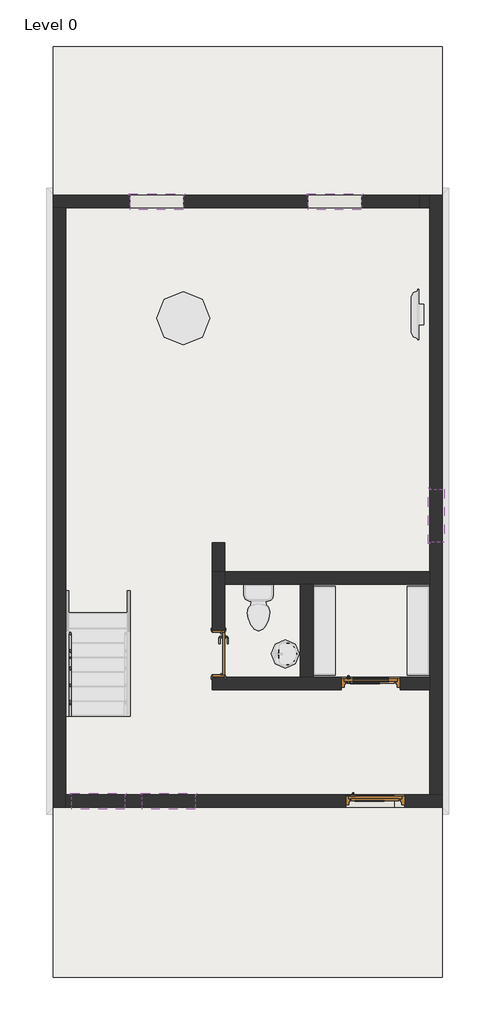
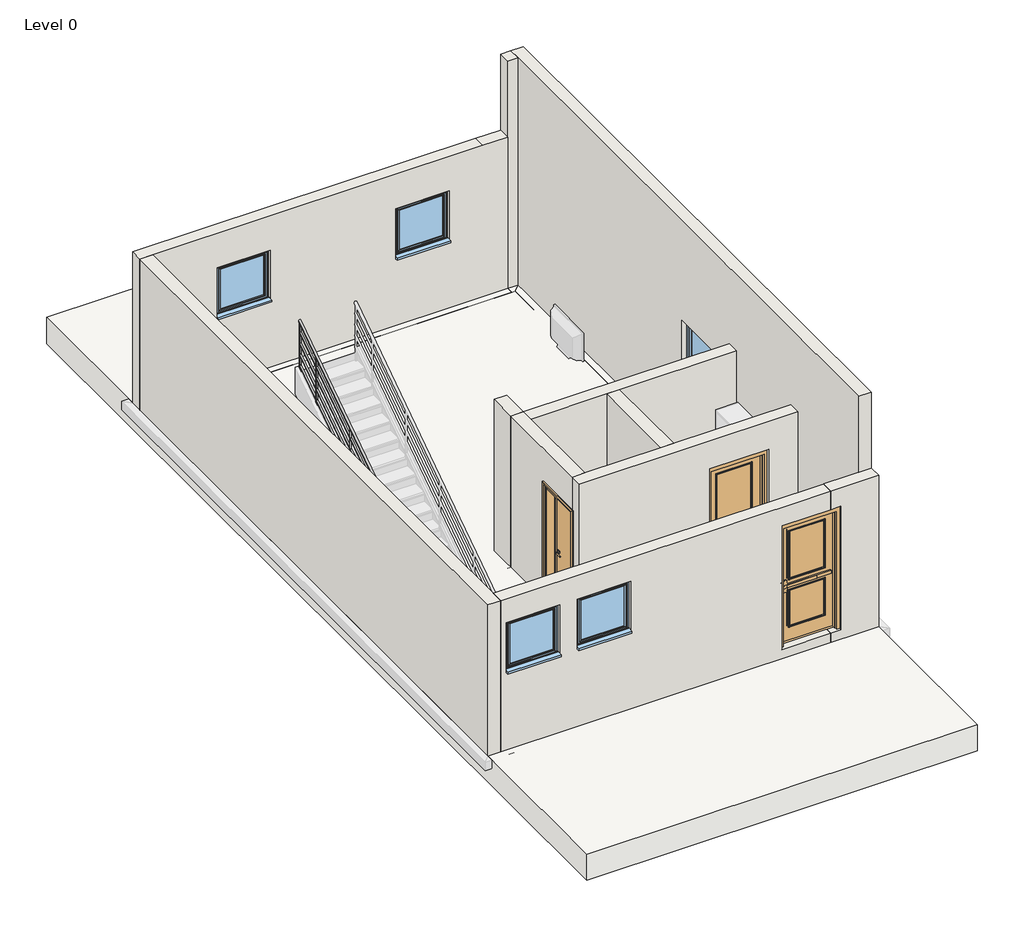
# One storey, part 1 of 2: 11 walls, 5 windows, 3 doors, 1 railing, 1 slab.
"""IFC4 building model written with IfcOpenShell, lengths in millimetres."""

from ifc_helpers import new_model, si_unit, frame, origin, origin_with_axes, place, context, project, spatial, polyline, circle_curve, ellipse_curve, outline, extrude, faceted_brep, transform, mapped, element, save
from ifc_brep_helpers import plane_surface, cylinder_surface, advanced_brep
from components import door_exterior_single_two_lite_door_exterior_single_two_lite_fa13afaf, doors_intsgl_810x2110mm_df607d29, windows_sgl_plain_910x910mm_6bfcc678

model = new_model("IFC4")

# Units and contexts
model_context = context("Model", 3, world=origin())
ifc_project = project(units=[si_unit("LENGTHUNIT", "METRE", prefix="MILLI")], contexts=[model_context])

# Site, building, storey
site = spatial("IfcSite", under=ifc_project)
building = spatial("IfcBuilding", under=site)
storey = spatial("IfcBuildingStorey", under=building, Name="Level 0", Elevation=0.0)

# Doors
placement = place(None, origin())
door_exterior_single_two_lite_door_exterior_single_two_lite_shape = door_exterior_single_two_lite_door_exterior_single_two_lite_fa13afaf(model_context)
element("IfcDoor", 1, ObjectType="Door-Exterior-Single-Two_Lite : Door-Exterior-Single-Two_Lite", at=placement, inside=storey, context=model_context, shape_type="MappedRepresentation", body=[
    mapped(door_exterior_single_two_lite_door_exterior_single_two_lite_shape, transform((-1402.2000057, 8728.6490528, 166.4), x_axis=(1.0, 0.0, 0.0), y_axis=(0.0, 1.0, 0.0), z_axis=(0.0, 0.0, 1.0))),
])
element("IfcDoor", 2, ObjectType="Door-Exterior-Single-Two_Lite : Door-Exterior-Single-Two_Lite", at=placement, inside=storey, context=model_context, shape_type="MappedRepresentation", body=[
    mapped(door_exterior_single_two_lite_door_exterior_single_two_lite_shape, transform((-1479.7250057, 10743.6490528, 0.0), x_axis=(1.0, 0.0, 0.0), y_axis=(0.0, 1.0, 0.0), z_axis=(0.0, 0.0, 1.0))),
])
doors_intsgl_810x2110mm_shape = doors_intsgl_810x2110mm_df607d29(model_context)
element("IfcDoor", 3, ObjectType="Doors_IntSgl : 810x2110mm", at=placement, inside=storey, context=model_context, shape_type="MappedRepresentation", body=[
    mapped(doors_intsgl_810x2110mm_shape, transform((-4092.7000057, 11262.4990528, 0.0), x_axis=(0.0, -1.0, 0.0), y_axis=(1.0, 0.0, 0.0), z_axis=(0.0, 0.0, 1.0))),
])

# Railing
element("IfcRailing", 4, ObjectType="900mm_Pipe", at=placement, inside=storey, context=model_context, shape_type="AdvancedBrep", body=[
    advanced_brep(
    [(-6614.8000057, 10192.4990528, 1044.3059087), (-6654.8000057, 10192.4990528, 1044.3059087), (-6614.8000057, 14692.4990528, 4075.8848561), (-6654.8000057, 14692.4990528, 4075.8848561)],
    [
        (0, 1, ellipse_curve(frame((-6634.8000057, 10192.4990528, 1044.3059087), z_axis=(0.0, -1.0, 0.0), x_axis=(0.0, 0.0, -1.0)), 24.1151439, 20.0)),
        (1, 0, ellipse_curve(frame((-6634.8000057, 10192.4990528, 1044.3059087), z_axis=(0.0, -1.0, 0.0), x_axis=(0.0, 0.0, -1.0)), 24.1151439, 20.0)),
        (2, 3, ellipse_curve(frame((-6634.8000057, 14692.4990528, 4075.8848561), z_axis=(0.0, 1.0, 0.0), x_axis=(0.0, 0.0, -1.0)), 24.1151439, 20.0)),
        (3, 2, ellipse_curve(frame((-6634.8000057, 14692.4990528, 4075.8848561), z_axis=(0.0, 1.0, 0.0), x_axis=(0.0, 0.0, -1.0)), 24.1151439, 20.0)),
        (0, 2),
        (3, 1),
    ],
    [
        plane_surface(frame((-6634.8000057, 10192.4990528, 1068.4210526), z_axis=(0.0, -1.0, 0.0), x_axis=(0.0, 0.0, 1.0))),
        plane_surface(frame((-6634.8000057, 14692.4990528, 4100.0), z_axis=(0.0, 1.0, 0.0), x_axis=(0.0, 0.0, 1.0))),
        cylinder_surface(frame((-6634.8000057, 10203.6735117, 1051.8339652), z_axis=(0.0, -0.8293543703358371, -0.5587229442262482), x_axis=(-1.0, 0.0, 0.0)), 20.0),
    ],
    [
        (0, [[1, 2]]),
        (1, [[3, 4]]),
        (2, [[-1, 5, -4, 6]]),
        (2, [[-2, -6, -3, -5]]),
    ],
),
    advanced_brep(
    [(-6619.8000057, 10192.4990528, 850.3346947), (-6649.8000057, 10192.4990528, 850.3346947), (-6619.8000057, 14692.4990528, 3881.9136421), (-6649.8000057, 14692.4990528, 3881.9136421)],
    [
        (0, 1, ellipse_curve(frame((-6634.8000057, 10192.4990528, 850.3346947), z_axis=(0.0, -1.0, 0.0), x_axis=(0.0, 0.0, -1.0)), 18.0863579, 15.0)),
        (1, 0, ellipse_curve(frame((-6634.8000057, 10192.4990528, 850.3346947), z_axis=(0.0, -1.0, 0.0), x_axis=(0.0, 0.0, -1.0)), 18.0863579, 15.0)),
        (2, 3, ellipse_curve(frame((-6634.8000057, 14692.4990528, 3881.9136421), z_axis=(0.0, 1.0, 0.0), x_axis=(0.0, 0.0, -1.0)), 18.0863579, 15.0)),
        (3, 2, ellipse_curve(frame((-6634.8000057, 14692.4990528, 3881.9136421), z_axis=(0.0, 1.0, 0.0), x_axis=(0.0, 0.0, -1.0)), 18.0863579, 15.0)),
        (0, 2),
        (3, 1),
    ],
    [
        plane_surface(frame((-6634.8000057, 10192.4990528, 868.4210526), z_axis=(0.0, -1.0, 0.0), x_axis=(0.0, 0.0, 1.0))),
        plane_surface(frame((-6634.8000057, 14692.4990528, 3900.0), z_axis=(0.0, 1.0, 0.0), x_axis=(0.0, 0.0, 1.0))),
        cylinder_surface(frame((-6634.8000057, 10200.879897, 855.9807371), z_axis=(0.0, -0.8293543703358371, -0.5587229442262482), x_axis=(-1.0, 0.0, 0.0)), 15.0),
    ],
    [
        (0, [[1, 2]]),
        (1, [[3, 4]]),
        (2, [[-1, 5, -4, 6]]),
        (2, [[-2, -6, -3, -5]]),
    ],
),
    advanced_brep(
    [(-6619.8000057, 10192.4990528, 650.3346947), (-6649.8000057, 10192.4990528, 650.3346947), (-6619.8000057, 14692.4990528, 3681.9136421), (-6649.8000057, 14692.4990528, 3681.9136421)],
    [
        (0, 1, ellipse_curve(frame((-6634.8000057, 10192.4990528, 650.3346947), z_axis=(0.0, -1.0, 0.0), x_axis=(0.0, 0.0, -1.0)), 18.0863579, 15.0)),
        (1, 0, ellipse_curve(frame((-6634.8000057, 10192.4990528, 650.3346947), z_axis=(0.0, -1.0, 0.0), x_axis=(0.0, 0.0, -1.0)), 18.0863579, 15.0)),
        (2, 3, ellipse_curve(frame((-6634.8000057, 14692.4990528, 3681.9136421), z_axis=(0.0, 1.0, 0.0), x_axis=(0.0, 0.0, -1.0)), 18.0863579, 15.0)),
        (3, 2, ellipse_curve(frame((-6634.8000057, 14692.4990528, 3681.9136421), z_axis=(0.0, 1.0, 0.0), x_axis=(0.0, 0.0, -1.0)), 18.0863579, 15.0)),
        (0, 2),
        (3, 1),
    ],
    [
        plane_surface(frame((-6634.8000057, 10192.4990528, 668.4210526), z_axis=(0.0, -1.0, 0.0), x_axis=(0.0, 0.0, 1.0))),
        plane_surface(frame((-6634.8000057, 14692.4990528, 3700.0), z_axis=(0.0, 1.0, 0.0), x_axis=(0.0, 0.0, 1.0))),
        cylinder_surface(frame((-6634.8000057, 10200.879897, 655.9807371), z_axis=(0.0, -0.8293543703358371, -0.5587229442262482), x_axis=(-1.0, 0.0, 0.0)), 15.0),
    ],
    [
        (0, [[1, 2]]),
        (1, [[3, 4]]),
        (2, [[-1, 5, -4, 6]]),
        (2, [[-2, -6, -3, -5]]),
    ],
),
    advanced_brep(
    [(-6619.8000057, 10192.4990528, 450.3346947), (-6649.8000057, 10192.4990528, 450.3346947), (-6619.8000057, 14692.4990528, 3481.9136421), (-6649.8000057, 14692.4990528, 3481.9136421)],
    [
        (0, 1, ellipse_curve(frame((-6634.8000057, 10192.4990528, 450.3346947), z_axis=(0.0, -1.0, 0.0), x_axis=(0.0, 0.0, -1.0)), 18.0863579, 15.0)),
        (1, 0, ellipse_curve(frame((-6634.8000057, 10192.4990528, 450.3346947), z_axis=(0.0, -1.0, 0.0), x_axis=(0.0, 0.0, -1.0)), 18.0863579, 15.0)),
        (2, 3, ellipse_curve(frame((-6634.8000057, 14692.4990528, 3481.9136421), z_axis=(0.0, 1.0, 0.0), x_axis=(0.0, 0.0, -1.0)), 18.0863579, 15.0)),
        (3, 2, ellipse_curve(frame((-6634.8000057, 14692.4990528, 3481.9136421), z_axis=(0.0, 1.0, 0.0), x_axis=(0.0, 0.0, -1.0)), 18.0863579, 15.0)),
        (0, 2),
        (3, 1),
    ],
    [
        plane_surface(frame((-6634.8000057, 10192.4990528, 468.4210526), z_axis=(0.0, -1.0, 0.0), x_axis=(0.0, 0.0, 1.0))),
        plane_surface(frame((-6634.8000057, 14692.4990528, 3500.0), z_axis=(0.0, 1.0, 0.0), x_axis=(0.0, 0.0, 1.0))),
        cylinder_surface(frame((-6634.8000057, 10200.879897, 455.9807371), z_axis=(0.0, -0.8293543703358371, -0.5587229442262482), x_axis=(-1.0, 0.0, 0.0)), 15.0),
    ],
    [
        (0, [[1, 2]]),
        (1, [[3, 4]]),
        (2, [[-1, 5, -4, 6]]),
        (2, [[-2, -6, -3, -5]]),
    ],
),
    advanced_brep(
    [(-6619.8000057, 10192.4990528, 250.3346947), (-6649.8000057, 10192.4990528, 250.3346947), (-6619.8000057, 14692.4990528, 3281.9136421), (-6649.8000057, 14692.4990528, 3281.9136421)],
    [
        (0, 1, ellipse_curve(frame((-6634.8000057, 10192.4990528, 250.3346947), z_axis=(0.0, -1.0, 0.0), x_axis=(0.0, 0.0, -1.0)), 18.0863579, 15.0)),
        (1, 0, ellipse_curve(frame((-6634.8000057, 10192.4990528, 250.3346947), z_axis=(0.0, -1.0, 0.0), x_axis=(0.0, 0.0, -1.0)), 18.0863579, 15.0)),
        (2, 3, ellipse_curve(frame((-6634.8000057, 14692.4990528, 3281.9136421), z_axis=(0.0, 1.0, 0.0), x_axis=(0.0, 0.0, -1.0)), 18.0863579, 15.0)),
        (3, 2, ellipse_curve(frame((-6634.8000057, 14692.4990528, 3281.9136421), z_axis=(0.0, 1.0, 0.0), x_axis=(0.0, 0.0, -1.0)), 18.0863579, 15.0)),
        (0, 2),
        (3, 1),
    ],
    [
        plane_surface(frame((-6634.8000057, 10192.4990528, 268.4210526), z_axis=(0.0, -1.0, 0.0), x_axis=(0.0, 0.0, 1.0))),
        plane_surface(frame((-6634.8000057, 14692.4990528, 3300.0), z_axis=(0.0, 1.0, 0.0), x_axis=(0.0, 0.0, 1.0))),
        cylinder_surface(frame((-6634.8000057, 10200.879897, 255.9807371), z_axis=(0.0, -0.8293543703358371, -0.5587229442262482), x_axis=(-1.0, 0.0, 0.0)), 15.0),
    ],
    [
        (0, [[1, 2]]),
        (1, [[3, 4]]),
        (2, [[-1, 5, -4, 6]]),
        (2, [[-2, -6, -3, -5]]),
    ],
),
    advanced_brep(
    [(-6647.3000057, 14192.4990528, 3714.9276069), (-6622.3000057, 14192.4990528, 3714.9276069), (-6622.3000057, 14192.4990528, 2863.1578947), (-6647.3000057, 14192.4990528, 2863.1578947)],
    [
        (0, 1, ellipse_curve(frame((-6634.8000057, 14192.4990528, 3714.9276069), z_axis=(0.0, 0.5587229442262482, -0.829354370335837), x_axis=(0.0, 0.8293543703358369, 0.5587229442262482)), 15.0719649, 12.5)),
        (1, 2),
        (2, 3, circle_curve(frame((-6634.8000057, 14192.4990528, 2863.1578947), z_axis=(0.0, 0.0, 1.0), x_axis=(1.0, 0.0, 0.0)), 12.5)),
        (3, 0),
        (3, 2, circle_curve(frame((-6634.8000057, 14192.4990528, 2863.1578947), z_axis=(0.0, 0.0, 1.0), x_axis=(1.0, 0.0, 0.0)), 12.5)),
        (1, 0, ellipse_curve(frame((-6634.8000057, 14192.4990528, 3714.9276069), z_axis=(0.0, 0.5587229442262482, -0.829354370335837), x_axis=(0.0, 0.8293543703358369, 0.5587229442262482)), 15.0719649, 12.5)),
    ],
    [
        cylinder_surface(frame((-6634.8000057, 14192.4990528, 2763.1578947), z_axis=(0.0, 0.0, 1.0), x_axis=(1.0, 0.0, 0.0)), 12.5),
        plane_surface(frame((-6609.8000057, 14217.4990528, 3731.7697122), z_axis=(0.0, -0.5587229442262482, 0.829354370335837), x_axis=(-1.0, 0.0, 0.0))),
        plane_surface(frame((-6609.8000057, 14167.4990528, 2863.1578947), z_axis=(0.0, 0.0, -1.0), x_axis=(-1.0, 0.0, 0.0))),
    ],
    [
        (0, [[1, 2, 3, 4]]),
        (0, [[5, -2, 6, -4]]),
        (1, [[-6, -1]]),
        (2, [[-5, -3]]),
    ],
),
    advanced_brep(
    [(-6647.3000057, 13192.4990528, 3041.2433964), (-6622.3000057, 13192.4990528, 3041.2433964), (-6622.3000057, 13192.4990528, 2189.4736842), (-6647.3000057, 13192.4990528, 2189.4736842)],
    [
        (0, 1, ellipse_curve(frame((-6634.8000057, 13192.4990528, 3041.2433964), z_axis=(0.0, 0.5587229442262482, -0.829354370335837), x_axis=(0.0, 0.8293543703358369, 0.5587229442262482)), 15.0719649, 12.5)),
        (1, 2),
        (2, 3, circle_curve(frame((-6634.8000057, 13192.4990528, 2189.4736842), z_axis=(0.0, 0.0, 1.0), x_axis=(1.0, 0.0, 0.0)), 12.5)),
        (3, 0),
        (3, 2, circle_curve(frame((-6634.8000057, 13192.4990528, 2189.4736842), z_axis=(0.0, 0.0, 1.0), x_axis=(1.0, 0.0, 0.0)), 12.5)),
        (1, 0, ellipse_curve(frame((-6634.8000057, 13192.4990528, 3041.2433964), z_axis=(0.0, 0.5587229442262482, -0.829354370335837), x_axis=(0.0, 0.8293543703358369, 0.5587229442262482)), 15.0719649, 12.5)),
    ],
    [
        cylinder_surface(frame((-6634.8000057, 13192.4990528, 2089.4736842), z_axis=(0.0, 0.0, 1.0), x_axis=(1.0, 0.0, 0.0)), 12.5),
        plane_surface(frame((-6609.8000057, 13217.4990528, 3058.0855016), z_axis=(0.0, -0.5587229442262482, 0.829354370335837), x_axis=(-1.0, 0.0, 0.0))),
        plane_surface(frame((-6609.8000057, 13167.4990528, 2189.4736842), z_axis=(0.0, 0.0, -1.0), x_axis=(-1.0, 0.0, 0.0))),
    ],
    [
        (0, [[1, 2, 3, 4]]),
        (0, [[5, -2, 6, -4]]),
        (1, [[-6, -1]]),
        (2, [[-5, -3]]),
    ],
),
    advanced_brep(
    [(-6647.3000057, 12192.4990528, 2367.5591858), (-6622.3000057, 12192.4990528, 2367.5591858), (-6622.3000057, 12192.4990528, 1515.7894737), (-6647.3000057, 12192.4990528, 1515.7894737)],
    [
        (0, 1, ellipse_curve(frame((-6634.8000057, 12192.4990528, 2367.5591858), z_axis=(0.0, 0.5587229442262482, -0.829354370335837), x_axis=(0.0, 0.8293543703358369, 0.5587229442262482)), 15.0719649, 12.5)),
        (1, 2),
        (2, 3, circle_curve(frame((-6634.8000057, 12192.4990528, 1515.7894737), z_axis=(0.0, 0.0, 1.0), x_axis=(1.0, 0.0, 0.0)), 12.5)),
        (3, 0),
        (3, 2, circle_curve(frame((-6634.8000057, 12192.4990528, 1515.7894737), z_axis=(0.0, 0.0, 1.0), x_axis=(1.0, 0.0, 0.0)), 12.5)),
        (1, 0, ellipse_curve(frame((-6634.8000057, 12192.4990528, 2367.5591858), z_axis=(0.0, 0.5587229442262482, -0.829354370335837), x_axis=(0.0, 0.8293543703358369, 0.5587229442262482)), 15.0719649, 12.5)),
    ],
    [
        cylinder_surface(frame((-6634.8000057, 12192.4990528, 1415.7894737), z_axis=(0.0, 0.0, 1.0), x_axis=(1.0, 0.0, 0.0)), 12.5),
        plane_surface(frame((-6609.8000057, 12217.4990528, 2384.4012911), z_axis=(0.0, -0.5587229442262482, 0.829354370335837), x_axis=(-1.0, 0.0, 0.0))),
        plane_surface(frame((-6609.8000057, 12167.4990528, 1515.7894737), z_axis=(0.0, 0.0, -1.0), x_axis=(-1.0, 0.0, 0.0))),
    ],
    [
        (0, [[1, 2, 3, 4]]),
        (0, [[5, -2, 6, -4]]),
        (1, [[-6, -1]]),
        (2, [[-5, -3]]),
    ],
),
    advanced_brep(
    [(-6647.3000057, 11192.4990528, 1693.8749753), (-6622.3000057, 11192.4990528, 1693.8749753), (-6622.3000057, 11192.4990528, 842.1052632), (-6647.3000057, 11192.4990528, 842.1052632)],
    [
        (0, 1, ellipse_curve(frame((-6634.8000057, 11192.4990528, 1693.8749753), z_axis=(0.0, 0.5587229442262482, -0.829354370335837), x_axis=(0.0, 0.8293543703358369, 0.5587229442262482)), 15.0719649, 12.5)),
        (1, 2),
        (2, 3, circle_curve(frame((-6634.8000057, 11192.4990528, 842.1052632), z_axis=(0.0, 0.0, 1.0), x_axis=(1.0, 0.0, 0.0)), 12.5)),
        (3, 0),
        (3, 2, circle_curve(frame((-6634.8000057, 11192.4990528, 842.1052632), z_axis=(0.0, 0.0, 1.0), x_axis=(1.0, 0.0, 0.0)), 12.5)),
        (1, 0, ellipse_curve(frame((-6634.8000057, 11192.4990528, 1693.8749753), z_axis=(0.0, 0.5587229442262482, -0.829354370335837), x_axis=(0.0, 0.8293543703358369, 0.5587229442262482)), 15.0719649, 12.5)),
    ],
    [
        cylinder_surface(frame((-6634.8000057, 11192.4990528, 742.1052632), z_axis=(0.0, 0.0, 1.0), x_axis=(1.0, 0.0, 0.0)), 12.5),
        plane_surface(frame((-6609.8000057, 11217.4990528, 1710.7170806), z_axis=(0.0, -0.5587229442262482, 0.829354370335837), x_axis=(-1.0, 0.0, 0.0))),
        plane_surface(frame((-6609.8000057, 11167.4990528, 842.1052632), z_axis=(0.0, 0.0, -1.0), x_axis=(-1.0, 0.0, 0.0))),
    ],
    [
        (0, [[1, 2, 3, 4]]),
        (0, [[5, -2, 6, -4]]),
        (1, [[-6, -1]]),
        (2, [[-5, -3]]),
    ],
),
    advanced_brep(
    [(-6647.3000057, 14679.9990528, 4043.3486595), (-6622.3000057, 14679.9990528, 4043.3486595), (-6622.3000057, 14679.9990528, 3031.5789474), (-6647.3000057, 14679.9990528, 3031.5789474)],
    [
        (0, 1, ellipse_curve(frame((-6634.8000057, 14679.9990528, 4043.3486595), z_axis=(0.0, 0.5587229442262482, -0.829354370335837), x_axis=(0.0, 0.8293543703358369, 0.5587229442262482)), 15.0719649, 12.5)),
        (1, 2),
        (2, 3, circle_curve(frame((-6634.8000057, 14679.9990528, 3031.5789474), z_axis=(0.0, 0.0, 1.0), x_axis=(1.0, 0.0, 0.0)), 12.5)),
        (3, 0),
        (3, 2, circle_curve(frame((-6634.8000057, 14679.9990528, 3031.5789474), z_axis=(0.0, 0.0, 1.0), x_axis=(1.0, 0.0, 0.0)), 12.5)),
        (1, 0, ellipse_curve(frame((-6634.8000057, 14679.9990528, 4043.3486595), z_axis=(0.0, 0.5587229442262482, -0.829354370335837), x_axis=(0.0, 0.8293543703358369, 0.5587229442262482)), 15.0719649, 12.5)),
    ],
    [
        cylinder_surface(frame((-6634.8000057, 14679.9990528, 2931.5789474), z_axis=(0.0, 0.0, 1.0), x_axis=(1.0, 0.0, 0.0)), 12.5),
        plane_surface(frame((-6609.8000057, 14704.9990528, 4060.1907648), z_axis=(0.0, -0.5587229442262482, 0.829354370335837), x_axis=(-1.0, 0.0, 0.0))),
        plane_surface(frame((-6609.8000057, 14654.9990528, 3031.5789474), z_axis=(0.0, 0.0, -1.0), x_axis=(-1.0, 0.0, 0.0))),
    ],
    [
        (0, [[1, 2, 3, 4]]),
        (0, [[5, -2, 6, -4]]),
        (1, [[-6, -1]]),
        (2, [[-5, -3]]),
    ],
),
    advanced_brep(
    [(-6647.3000057, 10204.9990528, 1028.6118174), (-6622.3000057, 10204.9990528, 1028.6118174), (-6622.3000057, 10204.9990528, 168.4210526), (-6647.3000057, 10204.9990528, 168.4210526)],
    [
        (0, 1, ellipse_curve(frame((-6634.8000057, 10204.9990528, 1028.6118174), z_axis=(0.0, 0.5587229442262482, -0.829354370335837), x_axis=(0.0, 0.8293543703358369, 0.5587229442262482)), 15.0719649, 12.5)),
        (1, 2),
        (2, 3, circle_curve(frame((-6634.8000057, 10204.9990528, 168.4210526), z_axis=(0.0, 0.0, 1.0), x_axis=(1.0, 0.0, 0.0)), 12.5)),
        (3, 0),
        (3, 2, circle_curve(frame((-6634.8000057, 10204.9990528, 168.4210526), z_axis=(0.0, 0.0, 1.0), x_axis=(1.0, 0.0, 0.0)), 12.5)),
        (1, 0, ellipse_curve(frame((-6634.8000057, 10204.9990528, 1028.6118174), z_axis=(0.0, 0.5587229442262482, -0.829354370335837), x_axis=(0.0, 0.8293543703358369, 0.5587229442262482)), 15.0719649, 12.5)),
    ],
    [
        cylinder_surface(frame((-6634.8000057, 10204.9990528, 68.4210526), z_axis=(0.0, 0.0, 1.0), x_axis=(1.0, 0.0, 0.0)), 12.5),
        plane_surface(frame((-6609.8000057, 10229.9990528, 1045.4539227), z_axis=(0.0, -0.5587229442262482, 0.829354370335837), x_axis=(-1.0, 0.0, 0.0))),
        plane_surface(frame((-6609.8000057, 10179.9990528, 168.4210526), z_axis=(0.0, 0.0, -1.0), x_axis=(-1.0, 0.0, 0.0))),
    ],
    [
        (0, [[1, 2, 3, 4]]),
        (0, [[5, -2, 6, -4]]),
        (1, [[-6, -1]]),
        (2, [[-5, -3]]),
    ],
),
])

# Slab
element("IfcSlab", 5, ObjectType="floor generic 150mm", at=placement, inside=storey, context=model_context, shape_type="SweptSolid", body=[
    extrude(outline(polyline([(-255.2000057, 21680.5260335), (-255.2000057, 5707.3361785), (-6925.2000057, 5707.3361785), (-6925.2000057, 21680.5260335), (-255.2000057, 21680.5260335)])), frame((0.0, 0.0, -470.0), z_axis=(0.0, 0.0, 1.0), x_axis=(1.0, 0.0, 0.0)), (0.0, 0.0, 1.0), 470.0),
])

# Walls
element("IfcWall", 6, ObjectType="Wall-Site_215Bwk_w-Footing", at=placement, inside=storey, context=model_context, shape_type="Brep", body=[
    faceted_brep([(-6925.2000057, 18917.4990528, 0.0), (-6710.2000057, 18917.4990528, 0.0), (-644.8785855, 18917.4990528, 0.0), (-644.8785855, 18917.4990528, 2730.0), (-1070.2000057, 18917.4990528, 2730.0), (-6710.2000057, 18917.4990528, 2730.0), (-6925.2000057, 18917.4990528, 2730.0), (-4700.2000057, 18917.4990528, 2110.0), (-4700.2000057, 18917.4990528, 1200.0), (-5610.2000057, 18917.4990528, 1200.0), (-5610.2000057, 18917.4990528, 2110.0), (-1644.8785855, 18917.4990528, 2110.0), (-1644.8785855, 18917.4990528, 1200.0), (-2554.8785855, 18917.4990528, 1200.0), (-2554.8785855, 18917.4990528, 2110.0), (-6925.2000057, 19132.4990528, 0.0), (-6925.2000057, 19132.4990528, 2730.0), (-1070.2000057, 19132.4990528, 2730.0), (-644.8785855, 19132.4990528, 2730.0), (-644.8785855, 19132.4990528, 0.0), (-4700.2000057, 19132.4990528, 2110.0), (-5610.2000057, 19132.4990528, 2110.0), (-5610.2000057, 19132.4990528, 1200.0), (-4700.2000057, 19132.4990528, 1200.0), (-1644.8785855, 19132.4990528, 2110.0), (-2554.8785855, 19132.4990528, 2110.0), (-2554.8785855, 19132.4990528, 1200.0), (-1644.8785855, 19132.4990528, 1200.0)], [[[0, 1, 2, 3, 4, 5, 6], [7, 8, 9, 10], [11, 12, 13, 14]], [[15, 16, 17, 18, 19], [20, 21, 22, 23], [24, 25, 26, 27]], [[2, 1, 0, 15, 19]], [[3, 2, 19, 18]], [[0, 6, 16, 15]], [[4, 3, 18, 17]], [[6, 5, 4, 17, 16]], [[8, 7, 20, 23]], [[9, 8, 23, 22]], [[10, 9, 22, 21]], [[7, 10, 21, 20]], [[12, 11, 24, 27]], [[13, 12, 27, 26]], [[14, 13, 26, 25]], [[11, 14, 25, 24]]]),
])
element("IfcWall", 7, ObjectType="Wall-Site_215Bwk_w-Footing", at=placement, inside=storey, context=model_context, shape_type="Brep", body=[
    faceted_brep([(-6710.2000057, 8627.4990528, 0.0), (-6710.2000057, 8842.4990528, 0.0), (-6710.2000057, 18917.4990528, 0.0), (-6710.2000057, 18917.4990528, 2730.0), (-6710.2000057, 14692.4990528, 2730.0), (-6710.2000057, 10192.4990528, 2730.0), (-6710.2000057, 8842.4990528, 2730.0), (-6710.2000057, 8627.4990528, 2730.0), (-6925.2000057, 8627.4990528, 0.0), (-6925.2000057, 8627.4990528, 2730.0), (-6925.2000057, 18917.4990528, 2730.0), (-6925.2000057, 18917.4990528, 0.0)], [[[0, 1, 2, 3, 4, 5, 6, 7]], [[8, 9, 10, 11]], [[2, 1, 0, 8, 11]], [[0, 7, 9, 8]], [[3, 2, 11, 10]], [[7, 6, 5, 4, 3, 10, 9]]]),
])
element("IfcWall", 8, ObjectType="Wall-Site_215Bwk_w-Footing", at=placement, inside=storey, context=model_context, shape_type="Brep", body=[
    faceted_brep([(-255.2000057, 8842.4990528, 0.0), (-470.2000057, 8842.4990528, 0.0), (-1075.2000057, 8842.4990528, 0.0), (-1075.2000057, 8842.4990528, 166.4), (-894.2000057, 8842.4990528, 166.4), (-894.2000057, 8842.4990528, 2401.6), (-1075.2000057, 8842.4990528, 2401.6), (-1075.2000057, 8842.4990528, 2730.0), (-1070.2000057, 8842.4990528, 2730.0), (-255.2000057, 8842.4990528, 2730.0), (-1075.2000057, 8627.4990528, 0.0), (-255.2000057, 8627.4990528, 0.0), (-255.2000057, 8627.4990528, 2730.0), (-1070.2000057, 8627.4990528, 2730.0), (-1075.2000057, 8627.4990528, 2730.0), (-1075.2000057, 8627.4990528, 2401.6), (-894.2000057, 8627.4990528, 2401.6), (-894.2000057, 8627.4990528, 166.4), (-1075.2000057, 8627.4990528, 166.4)], [[[0, 1, 2, 3, 4, 5, 6, 7, 8, 9]], [[10, 11, 12, 13, 14, 15, 16, 17, 18]], [[2, 1, 0, 11, 10]], [[14, 7, 6, 15]], [[2, 10, 18, 3]], [[0, 9, 12, 11]], [[12, 9, 8, 13]], [[8, 7, 14, 13]], [[4, 17, 16, 5]], [[5, 16, 15, 6]], [[17, 4, 3, 18]]]),
])
element("IfcWall", 9, ObjectType="Wall-Site_215Bwk_w-Footing", at=placement, inside=storey, context=model_context, shape_type="Brep", body=[
    faceted_brep([(-470.2000057, 19132.4990528, 0.0), (-470.2000057, 18917.4990528, 0.0), (-470.2000057, 12672.4990528, 0.0), (-470.2000057, 12457.4990528, 0.0), (-470.2000057, 10857.4990528, 0.0), (-470.2000057, 10642.4990528, 0.0), (-470.2000057, 8842.4990528, 0.0), (-470.2000057, 8842.4990528, 3200.0), (-470.2000057, 8842.4990528, 4100.0), (-470.2000057, 18917.4990528, 4100.0), (-470.2000057, 19132.4990528, 4100.0), (-470.2000057, 14082.4990528, 2300.0), (-470.2000057, 13172.4990528, 2300.0), (-470.2000057, 13172.4990528, 1390.0), (-470.2000057, 14082.4990528, 1390.0), (-255.2000057, 19132.4990528, 0.0), (-255.2000057, 19132.4990528, 4100.0), (-255.2000057, 8842.4990528, 4100.0), (-255.2000057, 8842.4990528, 2730.0), (-255.2000057, 8842.4990528, 0.0), (-255.2000057, 14082.4990528, 2300.0), (-255.2000057, 14082.4990528, 1390.0), (-255.2000057, 13172.4990528, 1390.0), (-255.2000057, 13172.4990528, 2300.0)], [[[0, 1, 2, 3, 4, 5, 6, 7, 8, 9, 10], [11, 12, 13, 14]], [[15, 16, 17, 18, 19], [20, 21, 22, 23]], [[6, 5, 4, 3, 2, 1, 0, 15, 19]], [[10, 9, 8, 17, 16]], [[0, 10, 16, 15]], [[21, 20, 11, 14]], [[22, 21, 14, 13]], [[23, 22, 13, 12]], [[20, 23, 12, 11]], [[6, 19, 18, 17, 8, 7]]]),
])
element("IfcWall", 10, ObjectType="Wall-Site_215Bwk_w-Footing", at=placement, inside=storey, context=model_context, shape_type="Brep", body=[
    faceted_brep([(-470.2000057, 10857.4990528, 2730.0), (-470.2000057, 10857.4990528, 0.0), (-971.7250057, 10857.4990528, 0.0), (-971.7250057, 10857.4990528, 2235.2), (-1987.7250057, 10857.4990528, 2235.2), (-1987.7250057, 10857.4990528, 0.0), (-2470.2000057, 10857.4990528, 0.0), (-2685.2000057, 10857.4990528, 0.0), (-4200.2000057, 10857.4990528, 0.0), (-4200.2000057, 10857.4990528, 2110.0), (-4200.2000057, 10857.4990528, 2730.0), (-3985.2000057, 10857.4990528, 2730.0), (-2685.2000057, 10857.4990528, 2730.0), (-2470.2000057, 10857.4990528, 2730.0), (-470.2000057, 10642.4990528, 0.0), (-470.2000057, 10642.4990528, 2730.0), (-4200.2000057, 10642.4990528, 2730.0), (-4200.2000057, 10642.4990528, 0.0), (-1987.7250057, 10642.4990528, 0.0), (-1987.7250057, 10642.4990528, 2235.2), (-971.7250057, 10642.4990528, 2235.2), (-971.7250057, 10642.4990528, 0.0)], [[[0, 1, 2, 3, 4, 5, 6, 7, 8, 9, 10, 11, 12, 13]], [[14, 15, 16, 17, 18, 19, 20, 21]], [[1, 14, 21, 2]], [[17, 8, 7, 6, 5, 18]], [[1, 0, 15, 14]], [[10, 9, 8, 17, 16]], [[0, 13, 12, 11, 10, 16, 15]], [[20, 3, 2, 21]], [[3, 20, 19, 4]], [[4, 19, 18, 5]]]),
])
element("IfcWall", 11, ObjectType="Wall-Site_215Bwk_w-Footing", at=placement, inside=storey, context=model_context, shape_type="Brep", body=[
    faceted_brep([(-3985.2000057, 12672.4990528, 0.0), (-3985.2000057, 12672.4990528, 2730.0), (-3985.2000057, 12457.4990528, 2730.0), (-3985.2000057, 10857.4990528, 2730.0), (-3985.2000057, 10857.4990528, 2110.0), (-3985.2000057, 11667.4990528, 2110.0), (-3985.2000057, 11667.4990528, 0.0), (-3985.2000057, 12457.4990528, 0.0), (-4200.2000057, 12672.4990528, 2730.0), (-4200.2000057, 12672.4990528, 0.0), (-4200.2000057, 11667.4990528, 0.0), (-4200.2000057, 11667.4990528, 2110.0), (-4200.2000057, 10857.4990528, 2110.0), (-4200.2000057, 10857.4990528, 2730.0)], [[[0, 1, 2, 3, 4, 5, 6, 7]], [[8, 9, 10, 11, 12, 13]], [[9, 0, 7, 6, 10]], [[3, 13, 12, 4]], [[1, 0, 9, 8]], [[3, 2, 1, 8, 13]], [[11, 5, 4, 12]], [[5, 11, 10, 6]]]),
])
element("IfcWall", 12, ObjectType="Wall-Site_215Bwk_w-Footing", at=placement, inside=storey, context=model_context, shape_type="Brep", body=[
    faceted_brep([(-3985.2000057, 12457.4990528, 0.0), (-2685.2000057, 12457.4990528, 0.0), (-2470.2000057, 12457.4990528, 0.0), (-470.2000057, 12457.4990528, 0.0), (-470.2000057, 12457.4990528, 2730.0), (-2470.2000057, 12457.4990528, 2730.0), (-2685.2000057, 12457.4990528, 2730.0), (-3985.2000057, 12457.4990528, 2730.0), (-3985.2000057, 12672.4990528, 0.0), (-3985.2000057, 12672.4990528, 2730.0), (-470.2000057, 12672.4990528, 2730.0), (-470.2000057, 12672.4990528, 0.0)], [[[0, 1, 2, 3, 4, 5, 6, 7]], [[8, 9, 10, 11]], [[3, 2, 1, 0, 8, 11]], [[0, 7, 9, 8]], [[4, 3, 11, 10]], [[7, 6, 5, 4, 10, 9]]]),
])
element("IfcWall", 13, ObjectType="Wall-Site_215Bwk_w-Footing", at=placement, inside=storey, context=model_context, shape_type="SweptSolid", body=[
    extrude(outline(polyline([(-2685.2000057, 10857.4990528), (-2685.2000057, 12457.4990528), (-2470.2000057, 12457.4990528), (-2470.2000057, 10857.4990528), (-2685.2000057, 10857.4990528)])), origin_with_axes(), (0.0, 0.0, 1.0), 2730.0),
])
element("IfcWall", 14, ObjectType="Wall-Site_215Bwk_w-Footing", at=placement, inside=storey, context=model_context, shape_type="SweptSolid", body=[
    extrude(outline(polyline([(-3985.2000057, 13164.9990528), (-3985.2000057, 12672.4990528), (-4200.2000057, 12672.4990528), (-4200.2000057, 13164.9990528), (-3985.2000057, 13164.9990528)])), origin_with_axes(), (0.0, 0.0, 1.0), 2730.0),
])
element("IfcWall", 15, ObjectType="Wall-Site_215Bwk_w-Footing", at=placement, inside=storey, context=model_context, shape_type="SweptSolid", body=[
    extrude(outline(polyline([(0.0, -6710.2000057), (0.0, -1075.2000057), (166.4, -1075.2000057), (166.4, -1910.2000057), (2401.6, -1910.2000057), (2401.6, -1075.2000057), (2730.0, -1075.2000057), (2730.0, -6710.2000057), (0.0, -6710.2000057)]), holes=[polyline([(2300.0, -5700.2000057), (1390.0, -5700.2000057), (1390.0, -6610.2000057), (2300.0, -6610.2000057), (2300.0, -5700.2000057)]), polyline([(2300.0, -4490.2000057), (1390.0, -4490.2000057), (1390.0, -5400.2000057), (2300.0, -5400.2000057), (2300.0, -4490.2000057)])]), frame((0.0, 8627.4990528, 0.0), z_axis=(0.0, 1.0, 0.0), x_axis=(0.0, 0.0, 1.0)), (0.0, 0.0, 1.0), 215.0),
])
element("IfcWall", 16, ObjectType="Wall-Site_215Bwk_w-Footing", at=placement, inside=storey, context=model_context, shape_type="Brep", body=[
    faceted_brep([(-644.8785855, 18917.4990528, 0.0), (-470.2000057, 18917.4990528, 0.0), (-470.2000057, 18917.4990528, 4100.0), (-644.8785855, 18917.4990528, 4100.0), (-644.8785855, 18917.4990528, 2730.0), (-644.8785855, 19132.4990528, 0.0), (-644.8785855, 19132.4990528, 2730.0), (-644.8785855, 19132.4990528, 4100.0), (-470.2000057, 19132.4990528, 4100.0), (-470.2000057, 19132.4990528, 0.0)], [[[0, 1, 2, 3, 4]], [[5, 6, 7, 8, 9]], [[1, 0, 5, 9]], [[3, 2, 8, 7]], [[0, 4, 3, 7, 6, 5]], [[2, 1, 9, 8]]]),
])

# Windows
windows_sgl_plain_910x910mm_shape = windows_sgl_plain_910x910mm_6bfcc678(model_context)
element("IfcWindow", 17, ObjectType="Windows_Sgl_Plain : 910x910mm", at=placement, inside=storey, context=model_context, shape_type="MappedRepresentation", body=[
    mapped(windows_sgl_plain_910x910mm_shape, transform((-6155.2000057, 8743.4556206, 190.0), x_axis=(-1.0, 0.0, 0.0), y_axis=(0.0, -1.0, 0.0), z_axis=(0.0, 0.0, 1.0))),
])
element("IfcWindow", 18, ObjectType="Windows_Sgl_Plain : 910x910mm", at=placement, inside=storey, context=model_context, shape_type="MappedRepresentation", body=[
    mapped(windows_sgl_plain_910x910mm_shape, transform((-4945.2000057, 8743.4556206, 190.0), x_axis=(-1.0, 0.0, 0.0), y_axis=(0.0, -1.0, 0.0), z_axis=(0.0, 0.0, 1.0))),
])
element("IfcWindow", 19, ObjectType="Windows_Sgl_Plain : 910x910mm", at=placement, inside=storey, context=model_context, shape_type="MappedRepresentation", body=[
    mapped(windows_sgl_plain_910x910mm_shape, transform((-371.1565735, 13627.4990528, 190.0), x_axis=(0.0, -1.0, 0.0), y_axis=(1.0, 0.0, 0.0), z_axis=(0.0, 0.0, 1.0))),
])
element("IfcWindow", 20, ObjectType="Windows_Sgl_Plain : 910x910mm", at=placement, inside=storey, context=model_context, shape_type="MappedRepresentation", body=[
    mapped(windows_sgl_plain_910x910mm_shape, transform((-5155.2000057, 19033.4556206, 0.0), x_axis=(-1.0, 0.0, 0.0), y_axis=(0.0, -1.0, 0.0), z_axis=(0.0, 0.0, 1.0))),
])
element("IfcWindow", 21, ObjectType="Windows_Sgl_Plain : 910x910mm", at=placement, inside=storey, context=model_context, shape_type="MappedRepresentation", body=[
    mapped(windows_sgl_plain_910x910mm_shape, transform((-2099.8785855, 19033.4556206, 0.0), x_axis=(-1.0, 0.0, 0.0), y_axis=(0.0, -1.0, 0.0), z_axis=(0.0, 0.0, 1.0))),
])

save(model, "model.ifc")

# Revit data of these elements
# Type "Door-Exterior-Single-Two_Lite : Door-Exterior-Single-Two_Lite"
#   Type Mark = "46"
#   Assembly Code = "B2030100"
#   Analytic Construction = "Metal frame, double glass door"
#   Top Rail = 152.4 mm
#   Threshold Offset [instance default] = 12.7 mm
#   Threshold Length [instance default] = 1016 mm
#   Thickness = 44.45 mm
#   Thermal Resistance (R) = 0.242926 (m²·K)/W
#   Swing Angle [instance default] = 90.00°
#   Strike Height = 1016 mm
#   Stiles = 152.4 mm
#   Rough Width [instance default] = 1016 mm
#   Rough Height [instance default] = 2235.2 mm
#   MFOpeningHeight [instance default] = 101.6 mm
#   MFOpeningWidth [instance default] = 101.6 mm
#   Lock Rail = 190.5 mm
#   Heat Transfer Coefficient (U) = 4.11674 W/(m²·K)
#   Glass Thickness = 19.05 mm
#   Inset Calculate [instance default] = 101.6 mm
#   Masonry Inset [instance default] = 25.4 mm
#   Height = 2133.6 mm
#   Width = 914.4 mm
#   Masonry Frame Depth = 146.05 mm
#   Bottom Rail = 254 mm
#   Masonry Frame [instance default] = yes
#   Function = 1
#   Threshold [instance default] = yes
#   Dry Wall Frame [instance default] = no
#   Threshold Material = none
#   Panic Bar Material = Metal - Stainless Steel
#   Panel Material = Metal - Painted - Grey
#   Glass Stop Material = Metal - Painted - Grey
#   Exterior Pull Material = Metal - Stainless Steel
#   Frame Material = Metal - Painted - Grey
#   Visual Light Transmittance = 0
#   Solar Heat Gain Coefficient = 0
#   Wall Closure = (empty or 0)
# Type "Doors_IntSgl : 810x2110mm"
#   Construction Type Id = "MDOOR"
#   Type Mark = "42"
#   Type Comments = "Internal Single"
#   Operation = "SingleSwingRight"
#   Manufacturer = "Revit"
#   Keynote = "L20"
#   Description = "Internal Single Door"
#   Analytic Construction = "Metal"
#   UnderCut = 8 mm
#   Tolerance = 2 mm
#   Thickness = 38 mm
#   Thermal Resistance (R) = 0.270117 (m²·K)/W
#   Structural Tolerance = 8 mm
#   StopDepth = 32 mm
#   Stop Thickness = 19 mm
#   Rough Width = 810 mm
#   Rough Height = 2110 mm
#   Height to Top Lock Rail = 1000 mm
#   Heat Transfer Coefficient (U) = 3.7021 W/(m²·K)
#   Handle Z Distance = 900 mm
#   Handle X Distance = 75 mm
#   Frame Thickness = 32 mm
#   Door Panel Width = 726 mm
#   Door Panel Thickness = 38 mm
#   Door Panel Offset = 0 mm
#   Height = 2110 mm
#   Width = 810 mm
#   Door Panel Height = 2060 mm
#   Architrave Setback = 5 mm
#   Define Thermal Properties by = 1
#   Vis - Ironmongery = yes
#   Material Ironmongery = Door - Handle
#   Material Frame = Door - Frame/Mullion (1)
#   Material Door = Door - Panel
#   Material Architrave = Door - Architrave
#   Visual Light Transmittance = 0
#   Solar Heat Gain Coefficient = 0
#   Function = (empty or 0)
#   Wall Closure = (empty or 0)
# Type "900mm_Pipe"
#   built-in parameter 1008612 = 0.019685 (stored number, unit not read)
#   built-in parameter 1008611 = 0.0984252 (stored number, unit not read)
#   built-in parameter 1008609 = 3.28084 (stored number, unit not read)
#   built-in parameter 1008604 = 0.19685 (stored number, unit not read)
#   built-in parameter 1008603 = 0.164042 (stored number, unit not read)
#   Railing Height = 900 mm
#   built-in parameter 1008630 = 2
#   built-in parameter 1008610 = 1
#   built-in parameter 1008605 = 1
#   built-in parameter 1008618 = Baluster_Round : 25mm
# Type "floor generic 150mm"
#   Keynote = "E60/130"
#   Function = 0
#   Layers, outside or top first: 65 mm "Concrete, Sand/Cement Screed" (function 4); 0 mm "Vapor Retarder" (function 100); 80 mm "Rigid insulation" (function 3); 150 mm "Air" (function 3); 0 mm "Damp-proofing" (function 100); 100 mm "Concrete Masonry, Floor Block" (function 1); 75 mm "Concrete, Precast" (function 1)
# Type "Wall-Site_215Bwk_w-Footing"
#   Keynote = "F10"
#   Layers, outside or top first: 215 mm "Brick, Engineering, Soldier Course" (function 1); 215 mm "Brick, Engineering" (function 1)
# Type "Windows_Sgl_Plain : 910x910mm"
#   Type Mark = "44"
#   Operation = "SinglePanel"
#   Construction Type Id = "SGL"
#   Manufacturer = "Revit"
#   Keynote = "L10"
#   Analytic Construction = "Large single-glazed windows"
#   Wrap Layers (Ext) from Ext = 102.5 mm
#   Wrap Layers (Int) from Ext = 177.5 mm
#   Window Board Projection = 25 mm
#   Window Board Extension = 25 mm
#   Visual Light Transmittance = 0.9
#   Solar Heat Gain Coefficient = 0.86
#   Rough Width = 910 mm
#   Rough Height = 910 mm
#   Height = 910 mm
#   Width = 910 mm
#   Heat Transfer Coefficient (U) = 5.5617 W/(m²·K)
#   Glazing Thickness = 24 mm
#   FrameOffset - External = 50 mm
#   Frame Depth = 65 mm
#   Default Head Height = 2110 mm
#   Cill Depth = 87.5 mm
#   Cavity Closer Width = 50 mm
#   Cavity Closer Offset from Ext = 102.5 mm
#   Cavity Closer Depth = 85 mm
#   Define Thermal Properties by = 1
#   Vis - Cavity Closers = yes
#   Define Thermal Properties by = 1
#   Material Trim = Window Frame
#   Material Glass = Glass
#   Material Frame = Window Frame
#   Wall Closure = (empty or 0)
# Elements 1, 2 (IfcDoor, "Door-Exterior-Single-Two_Lite : Door-Exterior-Single-Two_Lite")
#   Threshold Offset = 12.7 mm
#   Threshold Length = 1016 mm
#   Swing Angle = 90.00°
#   Rough Width = 1016 mm
#   Rough Height = 2235.2 mm
#   Masonry Inset = 25.4 mm
#   MFOpeningWidth = 101.6 mm
#   MFOpeningHeight = 101.6 mm
#   Inset Calculate = 101.6 mm
#   Threshold = yes
#   Masonry Frame = yes
#   Dry Wall Frame = no
#   Phase Created = New Construction
#   Materials on its faces: "Metal - Painted - Grey", "Metal - Stainless Steel", "Glass", "Door - Frame/Mullion"
# Element 3 (IfcDoor, "Doors_IntSgl : 810x2110mm")
#   Phase Created = New Construction
#   Materials on its faces: "Door - Architrave", "Door - Handle", "Door - Frame/Mullion (1)", "Door - Panel"
# Element 4 (IfcRailing, "900mm_Pipe")
#   Phase Created = New Construction
# Element 5 (IfcSlab, "floor generic 150mm")
#   Height Offset From Level = 0 mm
#   Phase Created = New Construction
#   Materials on its faces: "Concrete, Precast", "Concrete, Sand/Cement Screed"
# Elements 6, 10, 11, 12, 13, 15 (IfcWall, "Wall-Site_215Bwk_w-Footing")
#   Top Offset = 0 mm
#   Base Offset = 0 mm
#   wall height = 2730 mm
#   Phase Created = New Construction
#   Base Constraint = Level 0
#   Top Constraint = Level 1
#   Materials on its faces: "Brick, Engineering, Soldier Course", "Brick, Engineering"
# Elements 7, 14 (IfcWall, "Wall-Site_215Bwk_w-Footing")
#   Top Offset = 0 mm
#   Base Offset = 0 mm
#   wall height = 2730 mm
#   Phase Created = New Construction
#   Base Constraint = Level 0
#   Top Constraint = Level 1
#   Materials on its faces: "Brick, Engineering", "Brick, Engineering, Soldier Course"
# Element 8 (IfcWall, "Wall-Site_215Bwk_w-Footing")
#   Top Offset = 900 mm
#   Base Offset = 0 mm
#   wall height = 2730 mm
#   Phase Created = New Construction
#   Base Constraint = Level 0
#   Top Constraint = Level 1
#   Materials on its faces: "Brick, Engineering, Soldier Course", "Brick, Engineering"
# Element 9 (IfcWall, "Wall-Site_215Bwk_w-Footing")
#   Top Offset = 900 mm
#   Base Offset = 0 mm
#   wall height = 4100 mm
#   Phase Created = New Construction
#   Base Constraint = Level 0
#   Top Constraint = Level 1
#   Materials on its faces: "Brick, Engineering, Soldier Course", "Brick, Engineering", "Concrete, Cast In Situ"
# Element 16 (IfcWall, "Wall-Site_215Bwk_w-Footing")
#   Top Offset = 900 mm
#   Base Offset = 0 mm
#   wall height = 4100 mm
#   Phase Created = New Construction
#   Base Constraint = Level 0
#   Top Constraint = Level 1
#   Materials on its faces: "Brick, Engineering", "Brick, Engineering, Soldier Course"
# Element 17 (IfcWindow, "Windows_Sgl_Plain : 910x910mm")
#   Mark = "1"
#   Phase Created = New Construction
#   Materials on its faces: "Window Frame", "Glass"
# Element 18 (IfcWindow, "Windows_Sgl_Plain : 910x910mm")
#   Mark = "2"
#   Phase Created = New Construction
#   Materials on its faces: "Window Frame", "Glass"
# Element 19 (IfcWindow, "Windows_Sgl_Plain : 910x910mm")
#   Mark = "3"
#   Phase Created = New Construction
#   Materials on its faces: "Window Frame", "Glass"
# Element 20 (IfcWindow, "Windows_Sgl_Plain : 910x910mm")
#   Mark = "6"
#   Phase Created = New Construction
#   Materials on its faces: "Window Frame", "Glass"
# Element 21 (IfcWindow, "Windows_Sgl_Plain : 910x910mm")
#   Mark = "7"
#   Phase Created = New Construction
#   Materials on its faces: "Window Frame", "Glass"
# Materials
#   "Metal - Stainless Steel": class "Metal", colour RGB 247 247 247, transparency 0
#   "Metal - Painted - Grey": class "Paint", colour RGB 104 104 104, transparency 0
#   "Door - Handle": colour RGB 0 0 0, transparency 0, Keynote = "P21", Cost = 0
#   "Door - Frame/Mullion (1)": class "Wood", colour RGB 212 179 113, transparency 0, Keynote = "L20", Cost = 0
#   "Door - Panel": class "Wood", colour RGB 210 159 95, transparency 0, Keynote = "L20", Cost = 0
#   "Door - Architrave": class "Wood", colour RGB 154 90 5, transparency 0, Keynote = "P20", Cost = 0
#   "Concrete, Sand/Cement Screed": class "Concrete", colour RGB 127 127 127, transparency 0, Description = "Concrete slab topping", Cost = 0
#   "Vapor Retarder": class "Generic", colour RGB 120 120 120, transparency 0, Description = "Polyethylene film membrane", Cost = 0
#   "Rigid insulation": class "Generic", colour RGB 127 127 127, transparency 0, Description = "Rigid foam insulation board", Cost = 0
#   "Air": class "Gas", colour RGB 255 255 255, transparency 0, Description = "Air", Cost = 0
#   "Damp-proofing": class "Generic", colour RGB 127 127 127, transparency 0, Description = "Damp-proofing", Cost = 0
#   "Concrete Masonry, Floor Block": class "Concrete", colour RGB 181 181 181, transparency 0, Description = "physical material", Cost = 0
#   "Concrete, Precast": class "Concrete", colour RGB 192 192 192, transparency 0, Description = "Precast concrete", Cost = 0
#   "Brick, Engineering, Soldier Course": class "Masonry", colour RGB 102 147 188, transparency 0, Description = "High fired, dense brick", Cost = 0
#   "Brick, Engineering": class "Masonry", colour RGB 102 147 188, transparency 0, Description = "High fired, dense brick", Cost = 0
#   "Window Frame": colour RGB 249 249 249, transparency 0, Keynote = "L10", Cost = 0
#   "Glass": class "Glass", colour RGB 0 128 192, transparency 0.9, Description = "Soda Lime Glass", Cost = 0
#   "Door - Frame/Mullion": class "Wood", colour RGB 212 179 113, transparency 0, Keynote = "L20", Cost = 0
#   "Concrete, Cast In Situ": class "Concrete", colour RGB 192 192 192, transparency 0, Description = "physical material", Cost = 0
